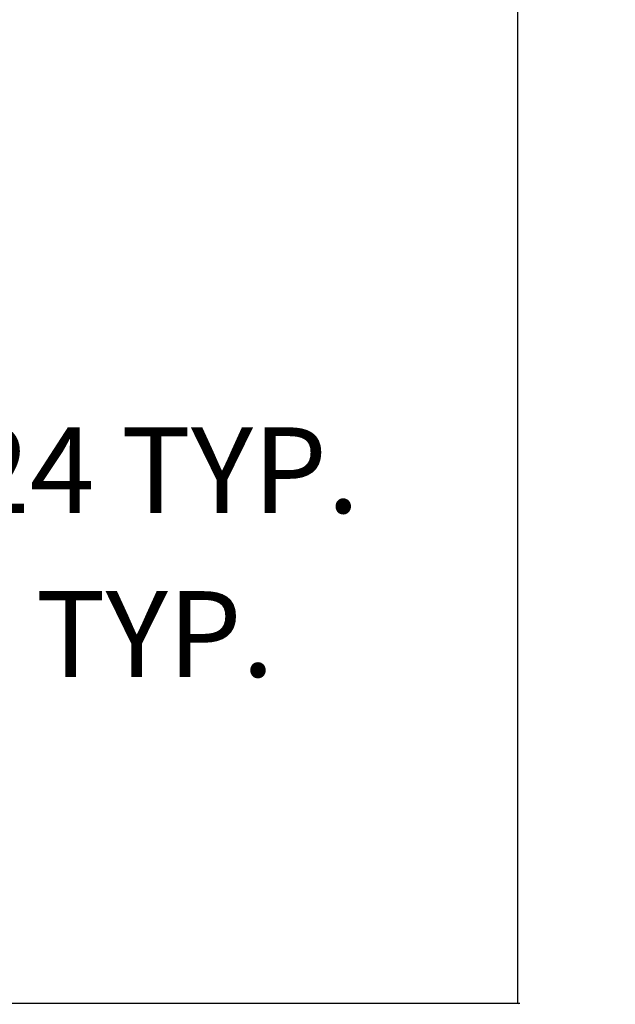
# Model space of a CAD drawing. Units: inches. Extents: x -48 to 50072, y 0 to 21068.
# Tile 39 of 75: x 555 to 611, y 214 to 306. Entities that reach past the tile are written whole.
import ezdxf

# ---------------------------------------------------------------- set-up
doc = ezdxf.new("R2010")
doc.units = ezdxf.units.IN
doc.header["$MEASUREMENT"] = 0
doc.layers.add('A-ANNO-DIMS', color=2, linetype='Continuous', lineweight=18)
doc.styles.get("Standard").update_dxf_attribs({"font": 'arial.ttf'})
doc.dimstyles.get("Standard").update_dxf_attribs({"dimtxt": 8, "dimasz": 0.18, "dimexe": 0.18, "dimexo": 0.0625, "dimgap": 0.09, "dimtad": 0, "dimtih": 1, "dimtoh": 1, "dimdec": 1, "dimzin": 0, "dimdsep": 46, "dimlunit": 4, "dimtxsty": 'Standard', "dimblk": 'ARCHTICK', "dimcen": 0.09, "dimadec": 0, "dimazin": 0, "dimtfac": 1, "dimtdec": 1, "dimtofl": 0, "dimtmove": 0, "dimatfit": 3, "dimldrblk": 'ARCHTICK', "dimfxl": 1, "dimtolj": 1, "dimtzin": 0, "dimarcsym": 0})

# ---------------------------------------------------------------- blocks, each defined once
blk = doc.blocks.new('_ArchTick')
at = {"color": 0, "linetype": 'ByBlock', "const_width": 0.15}
blk.add_lwpolyline([(-0.5, -0.5), (0.5, 0.5)], dxfattribs=at)
blk = doc.blocks.new('*D54')
at = {"layer": 'A-ANNO-DIMS', "color": 0, "lineweight": -2, "transparency": 16777216}
for p, q in [((540.551, 275.597), (544.198, 275.597)), ((544.018, 275.597), (544.018, 268.06)), ((544.018, 252.07), (544.018, 259.607)), ((540.551, 252.07), (544.198, 252.07))]:
    blk.add_line(p, q, dxfattribs=at)
at = {"layer": 'Defpoints', "color": 0, "transparency": 16777216}
for p in [(540.489, 275.597), (544.018, 275.597), (540.489, 252.07)]:
    blk.add_point(p, dxfattribs=at)
at = {"layer": 'A-ANNO-DIMS', "color": 0, "lineweight": -2, "transparency": 16777216, "xscale": 0.18, "yscale": 0.18, "zscale": 0.18}
for p, rotation in [((544.018, 275.597), 90), ((544.018, 252.07), 270)]:
    blk.add_blockref('_ArchTick', p, dxfattribs=dict(at, rotation=rotation))
at = {"layer": 'A-ANNO-DIMS', "color": 0, "transparency": 16777216, "insert": (544.018, 263.834), "char_height": 8, "attachment_point": 5}
blk.add_mtext('\\A1;SHRUB B 24 TYP.', dxfattribs=at)
blk = doc.blocks.new('*D55')
at = {"layer": 'A-ANNO-DIMS', "color": 0, "lineweight": -2, "transparency": 16777216}
for p, q in [((519.098, 252.008), (519.098, 248.361)), ((540.489, 252.008), (540.489, 248.361)), ((519.098, 248.541), (540.489, 248.541)), ((540.489, 248.541), (540.669, 248.541))]:
    blk.add_line(p, q, dxfattribs=at)
at = {"layer": 'Defpoints', "color": 0, "transparency": 16777216}
for p in [(519.098, 252.07), (540.489, 252.07), (540.489, 248.541)]:
    blk.add_point(p, dxfattribs=at)
at = {"layer": 'A-ANNO-DIMS', "color": 0, "lineweight": -2, "transparency": 16777216, "xscale": 0.18, "yscale": 0.18, "zscale": 0.18, "rotation": 180}
blk.add_blockref('_ArchTick', (519.098, 248.541), dxfattribs=at)
at = {"layer": 'A-ANNO-DIMS', "color": 0, "lineweight": -2, "transparency": 16777216, "xscale": 0.18, "yscale": 0.18, "zscale": 0.18}
blk.add_blockref('_ArchTick', (540.489, 248.541), dxfattribs=at)
at = {"layer": 'A-ANNO-DIMS', "color": 0, "transparency": 16777216, "insert": (560.298, 248.541), "char_height": 8, "attachment_point": 5}
blk.add_mtext('\\A1;21 TYP.', dxfattribs=at)
blk = doc.blocks.new('*D115')
at = {"layer": 'A-ANNO-DIMS', "color": 0, "lineweight": -2, "transparency": 16777216}
for p, q in [((549.08, 451.075), (601.647, 451.075)), ((601.467, 451.075), (601.467, 336.752)), ((601.467, 214.075), (601.467, 328.397)), ((553.58, 214.075), (601.647, 214.075))]:
    blk.add_line(p, q, dxfattribs=at)
at = {"layer": 'Defpoints', "color": 0, "transparency": 16777216}
for p in [(549.017, 451.075), (601.467, 451.075), (553.517, 214.075)]:
    blk.add_point(p, dxfattribs=at)
at = {"layer": 'A-ANNO-DIMS', "color": 0, "lineweight": -2, "transparency": 16777216, "xscale": 0.18, "yscale": 0.18, "zscale": 0.18}
for p, rotation in [((601.467, 451.075), 90), ((601.467, 214.075), 270)]:
    blk.add_blockref('_ArchTick', p, dxfattribs=dict(at, rotation=rotation))
at = {"layer": 'A-ANNO-DIMS', "color": 0, "transparency": 16777216, "insert": (601.467, 332.575), "char_height": 8, "attachment_point": 5}
blk.add_mtext('\\A1;237', dxfattribs=at)

msp = doc.modelspace()

# ---------------------------------------------------------------- dimensions: what is measured, and where the dimension line sits
at = {"layer": 'A-ANNO-DIMS'}
dim = msp.add_linear_dim(base=(601.467, 451.075), p1=(553.517, 214.075), p2=(549.017, 451.075), angle=90, dimstyle='Standard', override={"dimdec": 0, "dimlfac": 1, "dimrnd": 0, "dimzin": 0, "dimdsep": 46, "dimlunit": 2}, dxfattribs=at)
dim.commit()
dim.dimension.update_dxf_attribs({"geometry": '*D115', "text_midpoint": (601.467, 332.575)})
dim = msp.add_linear_dim(base=(544.018, 275.597), p1=(540.489, 252.07), p2=(540.489, 275.597), angle=90, text='SHRUB B <> TYP.', dimstyle='Standard', override={"dimdec": 0, "dimlfac": 1, "dimrnd": 0, "dimzin": 0, "dimdsep": 46, "dimlunit": 2}, dxfattribs=at)
dim.commit()
dim.dimension.update_dxf_attribs({"geometry": '*D54', "text_midpoint": (544.018, 263.834)})
dim = msp.add_linear_dim(base=(540.489, 248.541), p1=(519.098, 252.07), p2=(540.489, 252.07), text='<> TYP.', dimstyle='Standard', override={"dimdec": 0, "dimlfac": 1, "dimrnd": 0, "dimzin": 0, "dimdsep": 46, "dimlunit": 2}, dxfattribs=at)
dim.commit()
dim.dimension.update_dxf_attribs({"geometry": '*D55', "text_midpoint": (560.298, 248.541)})

doc.saveas('drawing.dxf')
